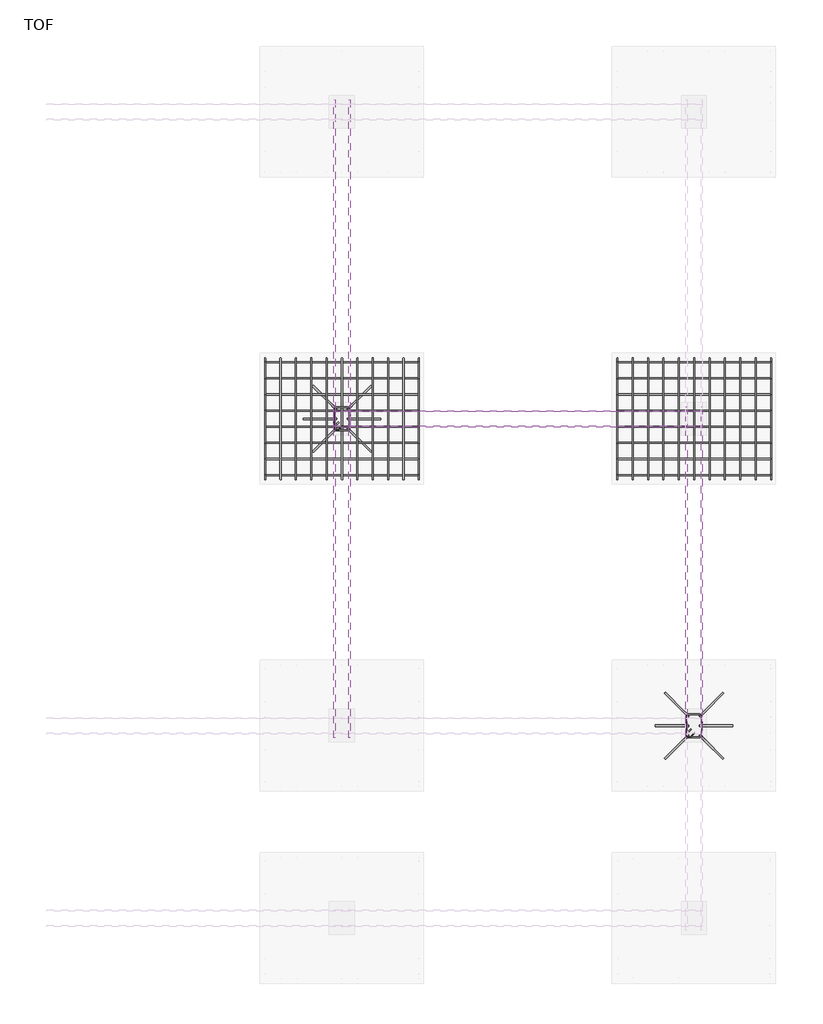
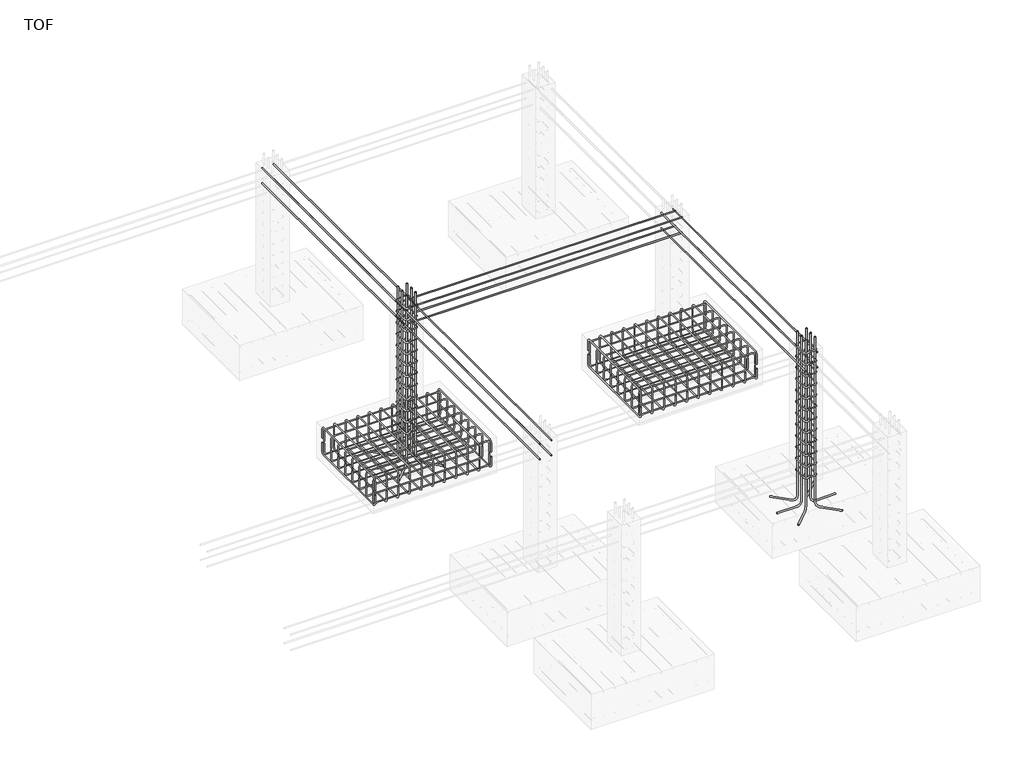
# One storey, part 8 of 10: 38 reinforcing bars.
"""IFC4 building model written with IfcOpenShell, lengths in millimetres."""

from ifc_helpers import new_model, si_unit, point, frame, origin, place, context, project, spatial, polyline, circle_curve, trimmed, segment, composite_curve, source, transform, mapped, element, save
from ifc_brep_helpers import swept_disk

model = new_model("IFC4")

# Units and contexts
model_context = context("Model", 3, world=origin())
ifc_project = project(units=[si_unit("LENGTHUNIT", "METRE", prefix="MILLI")], contexts=[model_context])

# Site, building, storey
site = spatial("IfcSite", under=ifc_project)
building = spatial("IfcBuilding", under=site)
storey = spatial("IfcBuildingStorey", under=building, Name="TOF", Elevation=-1828.8)

# Reinforcing bars
placement = place(None, origin())
reinforcing_bar_shape = source(origin(), model_context, "Body", "SolidModel", [
    swept_disk(composite_curve([segment(polyline([(10345.2782143, -9959.6267376, -2018.8), (10345.2782143, -9959.6267376, -1908.8)]), True, "CONTINUOUS"), segment(trimmed(circle_curve(frame((10345.2782143, -9994.6267376, -1908.8), z_axis=(1.0, 0.0, 0.0), x_axis=(0.0, 35.0, 0.0)), 35.0), [point((10345.2782143, -9959.6267376, -1908.8))], [point((10345.2782143, -9994.6267376, -1873.8))], True, "CARTESIAN"), True, "CONTINUOUS"), segment(polyline([(10345.2782143, -9994.6267376, -1873.8), (10345.2782143, -11034.6267376, -1873.8)]), True, "CONTINUOUS"), segment(trimmed(circle_curve(frame((10345.2782143, -11034.6267376, -1908.8), z_axis=(1.0, 0.0, 0.0), x_axis=(0.0, 0.0, 35.0)), 35.0), [point((10345.2782143, -11034.6267376, -1873.8))], [point((10345.2782143, -11069.6267376, -1908.8))], True, "CARTESIAN"), True, "CONTINUOUS"), segment(polyline([(10345.2782143, -11069.6267376, -1908.8), (10345.2782143, -11069.6267376, -2018.8)]), True, "CONTINUOUS")], self_intersect=False), 5.0),
])
element("IfcReinforcingBar", 1, at=placement, inside=storey, context=model_context, shape_type="MappedRepresentation", body=[
    mapped(reinforcing_bar_shape, transform((0.0, 0.0, 0.0), x_axis=(1.0, 0.0, 0.0), y_axis=(0.0, 1.0, 0.0), z_axis=(0.0, 0.0, 1.0))),
    mapped(reinforcing_bar_shape, transform((-141.0, 0.0, 0.0), x_axis=(1.0, 0.0, 0.0), y_axis=(0.0, 1.0, 0.0), z_axis=(0.0, 0.0, 1.0))),
    mapped(reinforcing_bar_shape, transform((-282.0, 0.0, 0.0), x_axis=(1.0, 0.0, 0.0), y_axis=(0.0, 1.0, 0.0), z_axis=(0.0, 0.0, 1.0))),
    mapped(reinforcing_bar_shape, transform((-423.0, 0.0, 0.0), x_axis=(1.0, 0.0, 0.0), y_axis=(0.0, 1.0, 0.0), z_axis=(0.0, 0.0, 1.0))),
    mapped(reinforcing_bar_shape, transform((-564.0, 0.0, 0.0), x_axis=(1.0, 0.0, 0.0), y_axis=(0.0, 1.0, 0.0), z_axis=(0.0, 0.0, 1.0))),
    mapped(reinforcing_bar_shape, transform((-705.0, 0.0, 0.0), x_axis=(1.0, 0.0, 0.0), y_axis=(0.0, 1.0, 0.0), z_axis=(0.0, 0.0, 1.0))),
    mapped(reinforcing_bar_shape, transform((-846.0, 0.0, 0.0), x_axis=(1.0, 0.0, 0.0), y_axis=(0.0, 1.0, 0.0), z_axis=(0.0, 0.0, 1.0))),
    mapped(reinforcing_bar_shape, transform((-987.0, 0.0, 0.0), x_axis=(1.0, 0.0, 0.0), y_axis=(0.0, 1.0, 0.0), z_axis=(0.0, 0.0, 1.0))),
    mapped(reinforcing_bar_shape, transform((-1128.0, 0.0, 0.0), x_axis=(1.0, 0.0, 0.0), y_axis=(0.0, 1.0, 0.0), z_axis=(0.0, 0.0, 1.0))),
    mapped(reinforcing_bar_shape, transform((-1269.0, 0.0, 0.0), x_axis=(1.0, 0.0, 0.0), y_axis=(0.0, 1.0, 0.0), z_axis=(0.0, 0.0, 1.0))),
    mapped(reinforcing_bar_shape, transform((-1410.0, 0.0, 0.0), x_axis=(1.0, 0.0, 0.0), y_axis=(0.0, 1.0, 0.0), z_axis=(0.0, 0.0, 1.0))),
])
reinforcing_bar_2_shape = source(origin(), model_context, "Body", "SolidModel", [
    swept_disk(composite_curve([segment(polyline([(10345.2782143, -11069.6267376, -2077.5233378), (10345.2782143, -11069.6267376, -2187.5233378)]), True, "CONTINUOUS"), segment(trimmed(circle_curve(frame((10345.2782143, -11034.6267376, -2187.5233378), z_axis=(1.0, 0.0, 0.0), x_axis=(0.0, -35.0, 0.0)), 35.0), [point((10345.2782143, -11069.6267376, -2187.5233378))], [point((10345.2782143, -11034.6267376, -2222.5233378))], True, "CARTESIAN"), True, "CONTINUOUS"), segment(polyline([(10345.2782143, -11034.6267376, -2222.5233378), (10345.2782143, -9994.6267376, -2222.5233378)]), True, "CONTINUOUS"), segment(trimmed(circle_curve(frame((10345.2782143, -9994.6267376, -2187.5233378), z_axis=(1.0, 0.0, 0.0), x_axis=(0.0, 0.0, -35.0)), 35.0), [point((10345.2782143, -9994.6267376, -2222.5233378))], [point((10345.2782143, -9959.6267376, -2187.5233378))], True, "CARTESIAN"), True, "CONTINUOUS"), segment(polyline([(10345.2782143, -9959.6267376, -2187.5233378), (10345.2782143, -9959.6267376, -2077.5233378)]), True, "CONTINUOUS")], self_intersect=False), 5.0),
])
element("IfcReinforcingBar", 2, at=placement, inside=storey, context=model_context, shape_type="MappedRepresentation", body=[
    mapped(reinforcing_bar_2_shape, transform((0.0, 0.0, 0.0), x_axis=(1.0, 0.0, 0.0), y_axis=(0.0, 1.0, 0.0), z_axis=(0.0, 0.0, 1.0))),
    mapped(reinforcing_bar_2_shape, transform((-141.0, 0.0, 0.0), x_axis=(1.0, 0.0, 0.0), y_axis=(0.0, 1.0, 0.0), z_axis=(0.0, 0.0, 1.0))),
    mapped(reinforcing_bar_2_shape, transform((-282.0, 0.0, 0.0), x_axis=(1.0, 0.0, 0.0), y_axis=(0.0, 1.0, 0.0), z_axis=(0.0, 0.0, 1.0))),
    mapped(reinforcing_bar_2_shape, transform((-423.0, 0.0, 0.0), x_axis=(1.0, 0.0, 0.0), y_axis=(0.0, 1.0, 0.0), z_axis=(0.0, 0.0, 1.0))),
    mapped(reinforcing_bar_2_shape, transform((-564.0, 0.0, 0.0), x_axis=(1.0, 0.0, 0.0), y_axis=(0.0, 1.0, 0.0), z_axis=(0.0, 0.0, 1.0))),
    mapped(reinforcing_bar_2_shape, transform((-705.0, 0.0, 0.0), x_axis=(1.0, 0.0, 0.0), y_axis=(0.0, 1.0, 0.0), z_axis=(0.0, 0.0, 1.0))),
    mapped(reinforcing_bar_2_shape, transform((-846.0, 0.0, 0.0), x_axis=(1.0, 0.0, 0.0), y_axis=(0.0, 1.0, 0.0), z_axis=(0.0, 0.0, 1.0))),
    mapped(reinforcing_bar_2_shape, transform((-987.0, 0.0, 0.0), x_axis=(1.0, 0.0, 0.0), y_axis=(0.0, 1.0, 0.0), z_axis=(0.0, 0.0, 1.0))),
    mapped(reinforcing_bar_2_shape, transform((-1128.0, 0.0, 0.0), x_axis=(1.0, 0.0, 0.0), y_axis=(0.0, 1.0, 0.0), z_axis=(0.0, 0.0, 1.0))),
    mapped(reinforcing_bar_2_shape, transform((-1269.0, 0.0, 0.0), x_axis=(1.0, 0.0, 0.0), y_axis=(0.0, 1.0, 0.0), z_axis=(0.0, 0.0, 1.0))),
    mapped(reinforcing_bar_2_shape, transform((-1410.0, 0.0, 0.0), x_axis=(1.0, 0.0, 0.0), y_axis=(0.0, 1.0, 0.0), z_axis=(0.0, 0.0, 1.0))),
])
reinforcing_bar_3_shape = source(origin(), model_context, "Body", "SolidModel", [
    swept_disk(composite_curve([segment(polyline([(10345.2782143, -9994.6861459, -2066.1776706), (10345.2782143, -9994.6861459, -2176.1776706)]), True, "CONTINUOUS"), segment(trimmed(circle_curve(frame((10310.2782143, -9994.6861459, -2176.1776706), z_axis=(0.0, 1.0, 0.0), x_axis=(35.0, 0.0, 0.0)), 35.0), [point((10345.2782143, -9994.6861459, -2176.1776706))], [point((10310.2782143, -9994.6861459, -2211.1776706))], True, "CARTESIAN"), True, "CONTINUOUS"), segment(polyline([(10310.2782143, -9994.6861459, -2211.1776706), (8970.2782143, -9994.6861459, -2211.1776706)]), True, "CONTINUOUS"), segment(trimmed(circle_curve(frame((8970.2782143, -9994.6861459, -2176.1776706), z_axis=(0.0, 1.0, 0.0), x_axis=(0.0, 0.0, -35.0)), 35.0), [point((8970.2782143, -9994.6861459, -2211.1776706))], [point((8935.2782143, -9994.6861459, -2176.1776706))], True, "CARTESIAN"), True, "CONTINUOUS"), segment(polyline([(8935.2782143, -9994.6861459, -2176.1776706), (8935.2782143, -9994.6861459, -2066.1776706)]), True, "CONTINUOUS")], self_intersect=False), 5.0),
])
element("IfcReinforcingBar", 3, at=placement, inside=storey, context=model_context, shape_type="MappedRepresentation", body=[
    mapped(reinforcing_bar_3_shape, transform((0.0, 0.0, 0.0), x_axis=(1.0, 0.0, 0.0), y_axis=(0.0, 1.0, 0.0), z_axis=(0.0, 0.0, 1.0))),
    mapped(reinforcing_bar_3_shape, transform((0.0, -148.0321606, 0.0), x_axis=(1.0, 0.0, 0.0), y_axis=(0.0, 1.0, 0.0), z_axis=(0.0, 0.0, 1.0))),
    mapped(reinforcing_bar_3_shape, transform((0.0, -296.0643211, 0.0), x_axis=(1.0, 0.0, 0.0), y_axis=(0.0, 1.0, 0.0), z_axis=(0.0, 0.0, 1.0))),
    mapped(reinforcing_bar_3_shape, transform((0.0, -444.0964817, 0.0), x_axis=(1.0, 0.0, 0.0), y_axis=(0.0, 1.0, 0.0), z_axis=(0.0, 0.0, 1.0))),
    mapped(reinforcing_bar_3_shape, transform((0.0, -592.1286423, 0.0), x_axis=(1.0, 0.0, 0.0), y_axis=(0.0, 1.0, 0.0), z_axis=(0.0, 0.0, 1.0))),
    mapped(reinforcing_bar_3_shape, transform((0.0, -740.1608029, 0.0), x_axis=(1.0, 0.0, 0.0), y_axis=(0.0, 1.0, 0.0), z_axis=(0.0, 0.0, 1.0))),
    mapped(reinforcing_bar_3_shape, transform((0.0, -888.1929634, 0.0), x_axis=(1.0, 0.0, 0.0), y_axis=(0.0, 1.0, 0.0), z_axis=(0.0, 0.0, 1.0))),
    mapped(reinforcing_bar_3_shape, transform((0.0, -1036.225124, 0.0), x_axis=(1.0, 0.0, 0.0), y_axis=(0.0, 1.0, 0.0), z_axis=(0.0, 0.0, 1.0))),
])
reinforcing_bar_4_shape = source(origin(), model_context, "Body", "SolidModel", [
    swept_disk(composite_curve([segment(polyline([(10345.2782143, -11030.9112699, -2039.256778), (10345.2782143, -11030.9112699, -1929.256778)]), True, "CONTINUOUS"), segment(trimmed(circle_curve(frame((10310.2782143, -11030.9112699, -1929.256778), z_axis=(0.0, -1.0, 0.0), x_axis=(35.0, 0.0, 0.0)), 35.0), [point((10345.2782143, -11030.9112699, -1929.256778))], [point((10310.2782143, -11030.9112699, -1894.256778))], True, "CARTESIAN"), True, "CONTINUOUS"), segment(polyline([(10310.2782143, -11030.9112699, -1894.256778), (8970.2782143, -11030.9112699, -1894.256778)]), True, "CONTINUOUS"), segment(trimmed(circle_curve(frame((8970.2782143, -11030.9112699, -1929.256778), z_axis=(0.0, -1.0, 0.0), x_axis=(0.0, 0.0, 35.0)), 35.0), [point((8970.2782143, -11030.9112699, -1894.256778))], [point((8935.2782143, -11030.9112699, -1929.256778))], True, "CARTESIAN"), True, "CONTINUOUS"), segment(polyline([(8935.2782143, -11030.9112699, -1929.256778), (8935.2782143, -11030.9112699, -2039.256778)]), True, "CONTINUOUS")], self_intersect=False), 5.0),
])
element("IfcReinforcingBar", 4, at=placement, inside=storey, context=model_context, shape_type="MappedRepresentation", body=[
    mapped(reinforcing_bar_4_shape, transform((0.0, 0.0, 0.0), x_axis=(1.0, 0.0, 0.0), y_axis=(0.0, 1.0, 0.0), z_axis=(0.0, 0.0, 1.0))),
    mapped(reinforcing_bar_4_shape, transform((0.0, 148.0321606, 0.0), x_axis=(1.0, 0.0, 0.0), y_axis=(0.0, 1.0, 0.0), z_axis=(0.0, 0.0, 1.0))),
    mapped(reinforcing_bar_4_shape, transform((0.0, 296.0643211, 0.0), x_axis=(1.0, 0.0, 0.0), y_axis=(0.0, 1.0, 0.0), z_axis=(0.0, 0.0, 1.0))),
    mapped(reinforcing_bar_4_shape, transform((0.0, 444.0964817, 0.0), x_axis=(1.0, 0.0, 0.0), y_axis=(0.0, 1.0, 0.0), z_axis=(0.0, 0.0, 1.0))),
    mapped(reinforcing_bar_4_shape, transform((0.0, 592.1286423, 0.0), x_axis=(1.0, 0.0, 0.0), y_axis=(0.0, 1.0, 0.0), z_axis=(0.0, 0.0, 1.0))),
    mapped(reinforcing_bar_4_shape, transform((0.0, 740.1608029, 0.0), x_axis=(1.0, 0.0, 0.0), y_axis=(0.0, 1.0, 0.0), z_axis=(0.0, 0.0, 1.0))),
    mapped(reinforcing_bar_4_shape, transform((0.0, 888.1929634, 0.0), x_axis=(1.0, 0.0, 0.0), y_axis=(0.0, 1.0, 0.0), z_axis=(0.0, 0.0, 1.0))),
    mapped(reinforcing_bar_4_shape, transform((0.0, 1036.225124, 0.0), x_axis=(1.0, 0.0, 0.0), y_axis=(0.0, 1.0, 0.0), z_axis=(0.0, 0.0, 1.0))),
])
reinforcing_bar_5_shape = source(origin(), model_context, "Body", "SolidModel", [
    swept_disk(composite_curve([segment(polyline([(13575.2782143, -9959.6267376, -2018.8), (13575.2782143, -9959.6267376, -1908.8)]), True, "CONTINUOUS"), segment(trimmed(circle_curve(frame((13575.2782143, -9994.6267376, -1908.8), z_axis=(1.0, 0.0, 0.0), x_axis=(0.0, 35.0, 0.0)), 35.0), [point((13575.2782143, -9959.6267376, -1908.8))], [point((13575.2782143, -9994.6267376, -1873.8))], True, "CARTESIAN"), True, "CONTINUOUS"), segment(polyline([(13575.2782143, -9994.6267376, -1873.8), (13575.2782143, -11034.6267376, -1873.8)]), True, "CONTINUOUS"), segment(trimmed(circle_curve(frame((13575.2782143, -11034.6267376, -1908.8), z_axis=(1.0, 0.0, 0.0), x_axis=(0.0, 0.0, 35.0)), 35.0), [point((13575.2782143, -11034.6267376, -1873.8))], [point((13575.2782143, -11069.6267376, -1908.8))], True, "CARTESIAN"), True, "CONTINUOUS"), segment(polyline([(13575.2782143, -11069.6267376, -1908.8), (13575.2782143, -11069.6267376, -2018.8)]), True, "CONTINUOUS")], self_intersect=False), 5.0),
])
element("IfcReinforcingBar", 5, at=placement, inside=storey, context=model_context, shape_type="MappedRepresentation", body=[
    mapped(reinforcing_bar_5_shape, transform((0.0, 0.0, 0.0), x_axis=(1.0, 0.0, 0.0), y_axis=(0.0, 1.0, 0.0), z_axis=(0.0, 0.0, 1.0))),
    mapped(reinforcing_bar_5_shape, transform((-141.0, 0.0, 0.0), x_axis=(1.0, 0.0, 0.0), y_axis=(0.0, 1.0, 0.0), z_axis=(0.0, 0.0, 1.0))),
    mapped(reinforcing_bar_5_shape, transform((-282.0, 0.0, 0.0), x_axis=(1.0, 0.0, 0.0), y_axis=(0.0, 1.0, 0.0), z_axis=(0.0, 0.0, 1.0))),
    mapped(reinforcing_bar_5_shape, transform((-423.0, 0.0, 0.0), x_axis=(1.0, 0.0, 0.0), y_axis=(0.0, 1.0, 0.0), z_axis=(0.0, 0.0, 1.0))),
    mapped(reinforcing_bar_5_shape, transform((-564.0, 0.0, 0.0), x_axis=(1.0, 0.0, 0.0), y_axis=(0.0, 1.0, 0.0), z_axis=(0.0, 0.0, 1.0))),
    mapped(reinforcing_bar_5_shape, transform((-705.0, 0.0, 0.0), x_axis=(1.0, 0.0, 0.0), y_axis=(0.0, 1.0, 0.0), z_axis=(0.0, 0.0, 1.0))),
    mapped(reinforcing_bar_5_shape, transform((-846.0, 0.0, 0.0), x_axis=(1.0, 0.0, 0.0), y_axis=(0.0, 1.0, 0.0), z_axis=(0.0, 0.0, 1.0))),
    mapped(reinforcing_bar_5_shape, transform((-987.0, 0.0, 0.0), x_axis=(1.0, 0.0, 0.0), y_axis=(0.0, 1.0, 0.0), z_axis=(0.0, 0.0, 1.0))),
    mapped(reinforcing_bar_5_shape, transform((-1128.0, 0.0, 0.0), x_axis=(1.0, 0.0, 0.0), y_axis=(0.0, 1.0, 0.0), z_axis=(0.0, 0.0, 1.0))),
    mapped(reinforcing_bar_5_shape, transform((-1269.0, 0.0, 0.0), x_axis=(1.0, 0.0, 0.0), y_axis=(0.0, 1.0, 0.0), z_axis=(0.0, 0.0, 1.0))),
    mapped(reinforcing_bar_5_shape, transform((-1410.0, 0.0, 0.0), x_axis=(1.0, 0.0, 0.0), y_axis=(0.0, 1.0, 0.0), z_axis=(0.0, 0.0, 1.0))),
])
reinforcing_bar_6_shape = source(origin(), model_context, "Body", "SolidModel", [
    swept_disk(composite_curve([segment(polyline([(13575.2782143, -11069.6267376, -2077.5233378), (13575.2782143, -11069.6267376, -2187.5233378)]), True, "CONTINUOUS"), segment(trimmed(circle_curve(frame((13575.2782143, -11034.6267376, -2187.5233378), z_axis=(1.0, 0.0, 0.0), x_axis=(0.0, -35.0, 0.0)), 35.0), [point((13575.2782143, -11069.6267376, -2187.5233378))], [point((13575.2782143, -11034.6267376, -2222.5233378))], True, "CARTESIAN"), True, "CONTINUOUS"), segment(polyline([(13575.2782143, -11034.6267376, -2222.5233378), (13575.2782143, -9994.6267376, -2222.5233378)]), True, "CONTINUOUS"), segment(trimmed(circle_curve(frame((13575.2782143, -9994.6267376, -2187.5233378), z_axis=(1.0, 0.0, 0.0), x_axis=(0.0, 0.0, -35.0)), 35.0), [point((13575.2782143, -9994.6267376, -2222.5233378))], [point((13575.2782143, -9959.6267376, -2187.5233378))], True, "CARTESIAN"), True, "CONTINUOUS"), segment(polyline([(13575.2782143, -9959.6267376, -2187.5233378), (13575.2782143, -9959.6267376, -2077.5233378)]), True, "CONTINUOUS")], self_intersect=False), 5.0),
])
element("IfcReinforcingBar", 6, at=placement, inside=storey, context=model_context, shape_type="MappedRepresentation", body=[
    mapped(reinforcing_bar_6_shape, transform((0.0, 0.0, 0.0), x_axis=(1.0, 0.0, 0.0), y_axis=(0.0, 1.0, 0.0), z_axis=(0.0, 0.0, 1.0))),
    mapped(reinforcing_bar_6_shape, transform((-141.0, 0.0, 0.0), x_axis=(1.0, 0.0, 0.0), y_axis=(0.0, 1.0, 0.0), z_axis=(0.0, 0.0, 1.0))),
    mapped(reinforcing_bar_6_shape, transform((-282.0, 0.0, 0.0), x_axis=(1.0, 0.0, 0.0), y_axis=(0.0, 1.0, 0.0), z_axis=(0.0, 0.0, 1.0))),
    mapped(reinforcing_bar_6_shape, transform((-423.0, 0.0, 0.0), x_axis=(1.0, 0.0, 0.0), y_axis=(0.0, 1.0, 0.0), z_axis=(0.0, 0.0, 1.0))),
    mapped(reinforcing_bar_6_shape, transform((-564.0, 0.0, 0.0), x_axis=(1.0, 0.0, 0.0), y_axis=(0.0, 1.0, 0.0), z_axis=(0.0, 0.0, 1.0))),
    mapped(reinforcing_bar_6_shape, transform((-705.0, 0.0, 0.0), x_axis=(1.0, 0.0, 0.0), y_axis=(0.0, 1.0, 0.0), z_axis=(0.0, 0.0, 1.0))),
    mapped(reinforcing_bar_6_shape, transform((-846.0, 0.0, 0.0), x_axis=(1.0, 0.0, 0.0), y_axis=(0.0, 1.0, 0.0), z_axis=(0.0, 0.0, 1.0))),
    mapped(reinforcing_bar_6_shape, transform((-987.0, 0.0, 0.0), x_axis=(1.0, 0.0, 0.0), y_axis=(0.0, 1.0, 0.0), z_axis=(0.0, 0.0, 1.0))),
    mapped(reinforcing_bar_6_shape, transform((-1128.0, 0.0, 0.0), x_axis=(1.0, 0.0, 0.0), y_axis=(0.0, 1.0, 0.0), z_axis=(0.0, 0.0, 1.0))),
    mapped(reinforcing_bar_6_shape, transform((-1269.0, 0.0, 0.0), x_axis=(1.0, 0.0, 0.0), y_axis=(0.0, 1.0, 0.0), z_axis=(0.0, 0.0, 1.0))),
    mapped(reinforcing_bar_6_shape, transform((-1410.0, 0.0, 0.0), x_axis=(1.0, 0.0, 0.0), y_axis=(0.0, 1.0, 0.0), z_axis=(0.0, 0.0, 1.0))),
])
reinforcing_bar_7_shape = source(origin(), model_context, "Body", "SolidModel", [
    swept_disk(composite_curve([segment(polyline([(13575.2782143, -9994.6861459, -2066.1776706), (13575.2782143, -9994.6861459, -2176.1776706)]), True, "CONTINUOUS"), segment(trimmed(circle_curve(frame((13540.2782143, -9994.6861459, -2176.1776706), z_axis=(0.0, 1.0, 0.0), x_axis=(35.0, 0.0, 0.0)), 35.0), [point((13575.2782143, -9994.6861459, -2176.1776706))], [point((13540.2782143, -9994.6861459, -2211.1776706))], True, "CARTESIAN"), True, "CONTINUOUS"), segment(polyline([(13540.2782143, -9994.6861459, -2211.1776706), (12200.2782143, -9994.6861459, -2211.1776706)]), True, "CONTINUOUS"), segment(trimmed(circle_curve(frame((12200.2782143, -9994.6861459, -2176.1776706), z_axis=(0.0, 1.0, 0.0), x_axis=(0.0, 0.0, -35.0)), 35.0), [point((12200.2782143, -9994.6861459, -2211.1776706))], [point((12165.2782143, -9994.6861459, -2176.1776706))], True, "CARTESIAN"), True, "CONTINUOUS"), segment(polyline([(12165.2782143, -9994.6861459, -2176.1776706), (12165.2782143, -9994.6861459, -2066.1776706)]), True, "CONTINUOUS")], self_intersect=False), 5.0),
])
element("IfcReinforcingBar", 7, at=placement, inside=storey, context=model_context, shape_type="MappedRepresentation", body=[
    mapped(reinforcing_bar_7_shape, transform((0.0, 0.0, 0.0), x_axis=(1.0, 0.0, 0.0), y_axis=(0.0, 1.0, 0.0), z_axis=(0.0, 0.0, 1.0))),
    mapped(reinforcing_bar_7_shape, transform((0.0, -148.0321606, 0.0), x_axis=(1.0, 0.0, 0.0), y_axis=(0.0, 1.0, 0.0), z_axis=(0.0, 0.0, 1.0))),
    mapped(reinforcing_bar_7_shape, transform((0.0, -296.0643211, 0.0), x_axis=(1.0, 0.0, 0.0), y_axis=(0.0, 1.0, 0.0), z_axis=(0.0, 0.0, 1.0))),
    mapped(reinforcing_bar_7_shape, transform((0.0, -444.0964817, 0.0), x_axis=(1.0, 0.0, 0.0), y_axis=(0.0, 1.0, 0.0), z_axis=(0.0, 0.0, 1.0))),
    mapped(reinforcing_bar_7_shape, transform((0.0, -592.1286423, 0.0), x_axis=(1.0, 0.0, 0.0), y_axis=(0.0, 1.0, 0.0), z_axis=(0.0, 0.0, 1.0))),
    mapped(reinforcing_bar_7_shape, transform((0.0, -740.1608029, 0.0), x_axis=(1.0, 0.0, 0.0), y_axis=(0.0, 1.0, 0.0), z_axis=(0.0, 0.0, 1.0))),
    mapped(reinforcing_bar_7_shape, transform((0.0, -888.1929634, 0.0), x_axis=(1.0, 0.0, 0.0), y_axis=(0.0, 1.0, 0.0), z_axis=(0.0, 0.0, 1.0))),
    mapped(reinforcing_bar_7_shape, transform((0.0, -1036.225124, 0.0), x_axis=(1.0, 0.0, 0.0), y_axis=(0.0, 1.0, 0.0), z_axis=(0.0, 0.0, 1.0))),
])
reinforcing_bar_8_shape = source(origin(), model_context, "Body", "SolidModel", [
    swept_disk(composite_curve([segment(polyline([(13575.2782143, -11030.9112699, -2039.256778), (13575.2782143, -11030.9112699, -1929.256778)]), True, "CONTINUOUS"), segment(trimmed(circle_curve(frame((13540.2782143, -11030.9112699, -1929.256778), z_axis=(0.0, -1.0, 0.0), x_axis=(35.0, 0.0, 0.0)), 35.0), [point((13575.2782143, -11030.9112699, -1929.256778))], [point((13540.2782143, -11030.9112699, -1894.256778))], True, "CARTESIAN"), True, "CONTINUOUS"), segment(polyline([(13540.2782143, -11030.9112699, -1894.256778), (12200.2782143, -11030.9112699, -1894.256778)]), True, "CONTINUOUS"), segment(trimmed(circle_curve(frame((12200.2782143, -11030.9112699, -1929.256778), z_axis=(0.0, -1.0, 0.0), x_axis=(0.0, 0.0, 35.0)), 35.0), [point((12200.2782143, -11030.9112699, -1894.256778))], [point((12165.2782143, -11030.9112699, -1929.256778))], True, "CARTESIAN"), True, "CONTINUOUS"), segment(polyline([(12165.2782143, -11030.9112699, -1929.256778), (12165.2782143, -11030.9112699, -2039.256778)]), True, "CONTINUOUS")], self_intersect=False), 5.0),
])
element("IfcReinforcingBar", 8, at=placement, inside=storey, context=model_context, shape_type="MappedRepresentation", body=[
    mapped(reinforcing_bar_8_shape, transform((0.0, 0.0, 0.0), x_axis=(1.0, 0.0, 0.0), y_axis=(0.0, 1.0, 0.0), z_axis=(0.0, 0.0, 1.0))),
    mapped(reinforcing_bar_8_shape, transform((0.0, 148.0321606, 0.0), x_axis=(1.0, 0.0, 0.0), y_axis=(0.0, 1.0, 0.0), z_axis=(0.0, 0.0, 1.0))),
    mapped(reinforcing_bar_8_shape, transform((0.0, 296.0643211, 0.0), x_axis=(1.0, 0.0, 0.0), y_axis=(0.0, 1.0, 0.0), z_axis=(0.0, 0.0, 1.0))),
    mapped(reinforcing_bar_8_shape, transform((0.0, 444.0964817, 0.0), x_axis=(1.0, 0.0, 0.0), y_axis=(0.0, 1.0, 0.0), z_axis=(0.0, 0.0, 1.0))),
    mapped(reinforcing_bar_8_shape, transform((0.0, 592.1286423, 0.0), x_axis=(1.0, 0.0, 0.0), y_axis=(0.0, 1.0, 0.0), z_axis=(0.0, 0.0, 1.0))),
    mapped(reinforcing_bar_8_shape, transform((0.0, 740.1608029, 0.0), x_axis=(1.0, 0.0, 0.0), y_axis=(0.0, 1.0, 0.0), z_axis=(0.0, 0.0, 1.0))),
    mapped(reinforcing_bar_8_shape, transform((0.0, 888.1929634, 0.0), x_axis=(1.0, 0.0, 0.0), y_axis=(0.0, 1.0, 0.0), z_axis=(0.0, 0.0, 1.0))),
    mapped(reinforcing_bar_8_shape, transform((0.0, 1036.225124, 0.0), x_axis=(1.0, 0.0, 0.0), y_axis=(0.0, 1.0, 0.0), z_axis=(0.0, 0.0, 1.0))),
])
reinforcing_bar_9_shape = source(origin(), model_context, "Body", "SolidModel", [
    swept_disk(composite_curve([segment(polyline([(12840.248777, -13360.7150493, -1784.8), (12806.3076515, -13394.6561748, -1784.8)]), True, "CONTINUOUS"), segment(trimmed(circle_curve(frame((12823.2782143, -13411.6267376, -1784.8), z_axis=(0.0, 0.0, 1.0), x_axis=(-16.970562800001062, 16.970562799999243, 0.0)), 24.0), [point((12806.3076515, -13394.6561748, -1784.8))], [point((12823.2782143, -13435.6267376, -1784.8))], True, "CARTESIAN"), True, "CONTINUOUS"), segment(polyline([(12823.2782143, -13435.6267376, -1784.8), (12917.2782143, -13435.6267376, -1784.8)]), True, "CONTINUOUS"), segment(trimmed(circle_curve(frame((12917.2782143, -13411.6267376, -1784.8), z_axis=(0.0, 0.0, 1.0), x_axis=(0.0, -24.0, 0.0)), 24.0), [point((12917.2782143, -13435.6267376, -1784.8))], [point((12941.2782143, -13411.6267376, -1784.8))], True, "CARTESIAN"), True, "CONTINUOUS"), segment(polyline([(12941.2782143, -13411.6267376, -1784.8), (12941.2782143, -13247.6267376, -1784.8)]), True, "CONTINUOUS"), segment(trimmed(circle_curve(frame((12917.3162115, -13247.6267376, -1786.149972), z_axis=(-0.05624883273897078, 0.0, 0.9984167811167355), x_axis=(23.962002800000846, 0.0, 1.3499719999999797)), 24.0), [point((12941.2782143, -13247.6267376, -1784.8))], [point((12917.3162115, -13223.6267376, -1786.149972))], True, "CARTESIAN"), True, "CONTINUOUS"), segment(polyline([(12917.3162115, -13223.6267376, -1786.149972), (12823.240217, -13223.6267376, -1791.450028)]), True, "CONTINUOUS"), segment(trimmed(circle_curve(frame((12823.240217, -13247.6267376, -1791.450028), z_axis=(-0.05624883273897078, 0.0, 0.9984167811167355), x_axis=(0.0, 24.0, 0.0)), 24.0), [point((12823.240217, -13223.6267376, -1791.450028))], [point((12799.2782143, -13247.6267376, -1792.8))], True, "CARTESIAN"), True, "CONTINUOUS"), segment(polyline([(12799.2782143, -13247.6267376, -1792.8), (12799.2782143, -13411.6267376, -1792.8)]), True, "CONTINUOUS"), segment(trimmed(circle_curve(frame((12823.2782143, -13411.6267376, -1792.8), z_axis=(0.0, 0.0, 1.0), x_axis=(-24.0, 0.0, 0.0)), 24.0), [point((12799.2782143, -13411.6267376, -1792.8))], [point((12840.248777, -13428.5973003, -1792.8))], True, "CARTESIAN"), True, "CONTINUOUS"), segment(polyline([(12840.248777, -13428.5973003, -1792.8), (12874.1899025, -13394.6561748, -1792.8)]), True, "CONTINUOUS")], self_intersect=False), 4.0),
])
element("IfcReinforcingBar", 9, at=placement, inside=storey, context=model_context, shape_type="MappedRepresentation", body=[
    mapped(reinforcing_bar_9_shape, transform((0.0, 0.0, 0.0), x_axis=(1.0, 0.0, 0.0), y_axis=(0.0, 1.0, 0.0), z_axis=(0.0, 0.0, 1.0))),
    mapped(reinforcing_bar_9_shape, transform((0.0, 0.0, 145.9395608), x_axis=(1.0, 0.0, 0.0), y_axis=(0.0, 1.0, 0.0), z_axis=(0.0, 0.0, 1.0))),
    mapped(reinforcing_bar_9_shape, transform((0.0, 0.0, 291.8791216), x_axis=(1.0, 0.0, 0.0), y_axis=(0.0, 1.0, 0.0), z_axis=(0.0, 0.0, 1.0))),
    mapped(reinforcing_bar_9_shape, transform((0.0, 0.0, 437.8186825), x_axis=(1.0, 0.0, 0.0), y_axis=(0.0, 1.0, 0.0), z_axis=(0.0, 0.0, 1.0))),
    mapped(reinforcing_bar_9_shape, transform((0.0, 0.0, 583.7582433), x_axis=(1.0, 0.0, 0.0), y_axis=(0.0, 1.0, 0.0), z_axis=(0.0, 0.0, 1.0))),
    mapped(reinforcing_bar_9_shape, transform((0.0, 0.0, 729.6978041), x_axis=(1.0, 0.0, 0.0), y_axis=(0.0, 1.0, 0.0), z_axis=(0.0, 0.0, 1.0))),
    mapped(reinforcing_bar_9_shape, transform((0.0, 0.0, 875.6373649), x_axis=(1.0, 0.0, 0.0), y_axis=(0.0, 1.0, 0.0), z_axis=(0.0, 0.0, 1.0))),
    mapped(reinforcing_bar_9_shape, transform((0.0, 0.0, 1021.5769258), x_axis=(1.0, 0.0, 0.0), y_axis=(0.0, 1.0, 0.0), z_axis=(0.0, 0.0, 1.0))),
    mapped(reinforcing_bar_9_shape, transform((0.0, 0.0, 1167.5164866), x_axis=(1.0, 0.0, 0.0), y_axis=(0.0, 1.0, 0.0), z_axis=(0.0, 0.0, 1.0))),
    mapped(reinforcing_bar_9_shape, transform((0.0, 0.0, 1313.4560474), x_axis=(1.0, 0.0, 0.0), y_axis=(0.0, 1.0, 0.0), z_axis=(0.0, 0.0, 1.0))),
    mapped(reinforcing_bar_9_shape, transform((0.0, 0.0, 1459.3956082), x_axis=(1.0, 0.0, 0.0), y_axis=(0.0, 1.0, 0.0), z_axis=(0.0, 0.0, 1.0))),
    mapped(reinforcing_bar_9_shape, transform((0.0, 0.0, 1605.3351691), x_axis=(1.0, 0.0, 0.0), y_axis=(0.0, 1.0, 0.0), z_axis=(0.0, 0.0, 1.0))),
])
element("IfcReinforcingBar", 10, at=placement, inside=storey, context=model_context, shape_type="SolidModel", body=[
    swept_disk(composite_curve([segment(polyline([(12925.884816, -13420.2333393, -20.0), (12925.884816, -13420.2333393, -2138.7824747)]), True, "CONTINUOUS"), segment(trimmed(circle_curve(frame((12965.1292424, -13459.4777657, -2138.7824747), z_axis=(-0.7071067811865545, -0.7071067811865406, 0.0), x_axis=(-39.24442640000052, 39.2444263999987, 0.0)), 55.5), [point((12925.884816, -13420.2333393, -2138.7824747))], [point((12965.1292424, -13459.4777657, -2194.2824747))], True, "CARTESIAN"), True, "CONTINUOUS"), segment(polyline([(12965.1292424, -13459.4777657, -2194.2824747), (13137.5083915, -13631.8569148, -2194.2824747)]), True, "CONTINUOUS")], self_intersect=False), 8.0),
])
element("IfcReinforcingBar", 11, at=placement, inside=storey, context=model_context, shape_type="SolidModel", body=[
    swept_disk(composite_curve([segment(polyline([(12925.934816, -13329.6267376, -20.0), (12925.934816, -13329.6267376, -2138.7824747)]), True, "CONTINUOUS"), segment(trimmed(circle_curve(frame((12981.434816, -13329.6267376, -2138.7824747), z_axis=(0.0, -1.0, 0.0), x_axis=(-55.5, 0.0, 0.0)), 55.5), [point((12925.934816, -13329.6267376, -2138.7824747))], [point((12981.434816, -13329.6267376, -2194.2824747))], True, "CARTESIAN"), True, "CONTINUOUS"), segment(polyline([(12981.434816, -13329.6267376, -2194.2824747), (13225.1657466, -13329.6267376, -2194.2824747)]), True, "CONTINUOUS")], self_intersect=False), 8.0),
])
element("IfcReinforcingBar", 12, at=placement, inside=storey, context=model_context, shape_type="SolidModel", body=[
    swept_disk(composite_curve([segment(polyline([(12925.884816, -13239.0201359, -20.0), (12925.884816, -13239.0201359, -2138.7824747)]), True, "CONTINUOUS"), segment(trimmed(circle_curve(frame((12965.1292424, -13199.7757095, -2138.7824747), z_axis=(0.7071067811865545, -0.7071067811865407, 0.0), x_axis=(-39.24442640000052, -39.24442640000052, 0.0)), 55.5), [point((12925.884816, -13239.0201359, -2138.7824747))], [point((12965.1292424, -13199.7757095, -2194.2824747))], True, "CARTESIAN"), True, "CONTINUOUS"), segment(polyline([(12965.1292424, -13199.7757095, -2194.2824747), (13137.5083915, -13027.3965603, -2194.2824747)]), True, "CONTINUOUS")], self_intersect=False), 8.0),
])
element("IfcReinforcingBar", 13, at=placement, inside=storey, context=model_context, shape_type="SolidModel", body=[
    swept_disk(composite_curve([segment(polyline([(12814.6716126, -13420.2333393, -20.0), (12814.6716126, -13420.2333393, -2138.7824747)]), True, "CONTINUOUS"), segment(trimmed(circle_curve(frame((12775.4271862, -13459.4777657, -2138.7824747), z_axis=(-0.7071067811865517, 0.7071067811865434, 0.0), x_axis=(39.2444263999987, 39.2444263999987, 0.0)), 55.5), [point((12814.6716126, -13420.2333393, -2138.7824747))], [point((12775.4271862, -13459.4777657, -2194.2824747))], True, "CARTESIAN"), True, "CONTINUOUS"), segment(polyline([(12775.4271862, -13459.4777657, -2194.2824747), (12603.048037, -13631.8569148, -2194.2824747)]), True, "CONTINUOUS")], self_intersect=False), 8.0),
])
element("IfcReinforcingBar", 14, at=placement, inside=storey, context=model_context, shape_type="SolidModel", body=[
    swept_disk(composite_curve([segment(polyline([(12814.6216126, -13329.6267376, -20.0), (12814.6216126, -13329.6267376, -2138.7824747)]), True, "CONTINUOUS"), segment(trimmed(circle_curve(frame((12759.1216126, -13329.6267376, -2138.7824747), z_axis=(0.0, 1.0, 0.0), x_axis=(55.5, 0.0, 0.0)), 55.5), [point((12814.6216126, -13329.6267376, -2138.7824747))], [point((12759.1216126, -13329.6267376, -2194.2824747))], True, "CARTESIAN"), True, "CONTINUOUS"), segment(polyline([(12759.1216126, -13329.6267376, -2194.2824747), (12515.3906819, -13329.6267376, -2194.2824747)]), True, "CONTINUOUS")], self_intersect=False), 8.0),
])
element("IfcReinforcingBar", 15, at=placement, inside=storey, context=model_context, shape_type="SolidModel", body=[
    swept_disk(composite_curve([segment(polyline([(12814.6716126, -13239.0201359, -20.0), (12814.6716126, -13239.0201359, -2138.7824747)]), True, "CONTINUOUS"), segment(trimmed(circle_curve(frame((12775.4271862, -13199.7757095, -2138.7824747), z_axis=(0.7071067811865572, 0.7071067811865379, 0.0), x_axis=(39.2444263999987, -39.24442640000052, 0.0)), 55.5), [point((12814.6716126, -13239.0201359, -2138.7824747))], [point((12775.4271862, -13199.7757095, -2194.2824747))], True, "CARTESIAN"), True, "CONTINUOUS"), segment(polyline([(12775.4271862, -13199.7757095, -2194.2824747), (12603.048037, -13027.3965603, -2194.2824747)]), True, "CONTINUOUS")], self_intersect=False), 8.0),
])
reinforcing_bar_10_shape = source(origin(), model_context, "Body", "SolidModel", [
    swept_disk(composite_curve([segment(polyline([(9610.248777, -10545.7150493, -1784.8), (9576.3076515, -10579.6561748, -1784.8)]), True, "CONTINUOUS"), segment(trimmed(circle_curve(frame((9593.2782143, -10596.6267376, -1784.8), z_axis=(0.0, 0.0, 1.0), x_axis=(-16.970562800001062, 16.970562799999243, 0.0)), 24.0), [point((9576.3076515, -10579.6561748, -1784.8))], [point((9593.2782143, -10620.6267376, -1784.8))], True, "CARTESIAN"), True, "CONTINUOUS"), segment(polyline([(9593.2782143, -10620.6267376, -1784.8), (9687.2782143, -10620.6267376, -1784.8)]), True, "CONTINUOUS"), segment(trimmed(circle_curve(frame((9687.2782143, -10596.6267376, -1784.8), z_axis=(0.0, 0.0, 1.0), x_axis=(0.0, -24.0, 0.0)), 24.0), [point((9687.2782143, -10620.6267376, -1784.8))], [point((9711.2782143, -10596.6267376, -1784.8))], True, "CARTESIAN"), True, "CONTINUOUS"), segment(polyline([(9711.2782143, -10596.6267376, -1784.8), (9711.2782143, -10432.6267376, -1784.8)]), True, "CONTINUOUS"), segment(trimmed(circle_curve(frame((9687.3162115, -10432.6267376, -1786.149972), z_axis=(-0.05624883273897078, 0.0, 0.9984167811167355), x_axis=(23.962002800000846, 0.0, 1.3499719999999797)), 24.0), [point((9711.2782143, -10432.6267376, -1784.8))], [point((9687.3162115, -10408.6267376, -1786.149972))], True, "CARTESIAN"), True, "CONTINUOUS"), segment(polyline([(9687.3162115, -10408.6267376, -1786.149972), (9593.240217, -10408.6267376, -1791.450028)]), True, "CONTINUOUS"), segment(trimmed(circle_curve(frame((9593.240217, -10432.6267376, -1791.450028), z_axis=(-0.05624883273897078, 0.0, 0.9984167811167355), x_axis=(0.0, 24.0, 0.0)), 24.0), [point((9593.240217, -10408.6267376, -1791.450028))], [point((9569.2782143, -10432.6267376, -1792.8))], True, "CARTESIAN"), True, "CONTINUOUS"), segment(polyline([(9569.2782143, -10432.6267376, -1792.8), (9569.2782143, -10596.6267376, -1792.8)]), True, "CONTINUOUS"), segment(trimmed(circle_curve(frame((9593.2782143, -10596.6267376, -1792.8), z_axis=(0.0, 0.0, 1.0), x_axis=(-24.0, 0.0, 0.0)), 24.0), [point((9569.2782143, -10596.6267376, -1792.8))], [point((9610.248777, -10613.5973003, -1792.8))], True, "CARTESIAN"), True, "CONTINUOUS"), segment(polyline([(9610.248777, -10613.5973003, -1792.8), (9644.1899025, -10579.6561748, -1792.8)]), True, "CONTINUOUS")], self_intersect=False), 4.0),
])
element("IfcReinforcingBar", 16, at=placement, inside=storey, context=model_context, shape_type="MappedRepresentation", body=[
    mapped(reinforcing_bar_10_shape, transform((0.0, 0.0, 0.0), x_axis=(1.0, 0.0, 0.0), y_axis=(0.0, 1.0, 0.0), z_axis=(0.0, 0.0, 1.0))),
    mapped(reinforcing_bar_10_shape, transform((0.0, 0.0, 145.9395608), x_axis=(1.0, 0.0, 0.0), y_axis=(0.0, 1.0, 0.0), z_axis=(0.0, 0.0, 1.0))),
    mapped(reinforcing_bar_10_shape, transform((0.0, 0.0, 291.8791216), x_axis=(1.0, 0.0, 0.0), y_axis=(0.0, 1.0, 0.0), z_axis=(0.0, 0.0, 1.0))),
    mapped(reinforcing_bar_10_shape, transform((0.0, 0.0, 437.8186825), x_axis=(1.0, 0.0, 0.0), y_axis=(0.0, 1.0, 0.0), z_axis=(0.0, 0.0, 1.0))),
    mapped(reinforcing_bar_10_shape, transform((0.0, 0.0, 583.7582433), x_axis=(1.0, 0.0, 0.0), y_axis=(0.0, 1.0, 0.0), z_axis=(0.0, 0.0, 1.0))),
    mapped(reinforcing_bar_10_shape, transform((0.0, 0.0, 729.6978041), x_axis=(1.0, 0.0, 0.0), y_axis=(0.0, 1.0, 0.0), z_axis=(0.0, 0.0, 1.0))),
    mapped(reinforcing_bar_10_shape, transform((0.0, 0.0, 875.6373649), x_axis=(1.0, 0.0, 0.0), y_axis=(0.0, 1.0, 0.0), z_axis=(0.0, 0.0, 1.0))),
    mapped(reinforcing_bar_10_shape, transform((0.0, 0.0, 1021.5769258), x_axis=(1.0, 0.0, 0.0), y_axis=(0.0, 1.0, 0.0), z_axis=(0.0, 0.0, 1.0))),
    mapped(reinforcing_bar_10_shape, transform((0.0, 0.0, 1167.5164866), x_axis=(1.0, 0.0, 0.0), y_axis=(0.0, 1.0, 0.0), z_axis=(0.0, 0.0, 1.0))),
    mapped(reinforcing_bar_10_shape, transform((0.0, 0.0, 1313.4560474), x_axis=(1.0, 0.0, 0.0), y_axis=(0.0, 1.0, 0.0), z_axis=(0.0, 0.0, 1.0))),
    mapped(reinforcing_bar_10_shape, transform((0.0, 0.0, 1459.3956082), x_axis=(1.0, 0.0, 0.0), y_axis=(0.0, 1.0, 0.0), z_axis=(0.0, 0.0, 1.0))),
    mapped(reinforcing_bar_10_shape, transform((0.0, 0.0, 1605.3351691), x_axis=(1.0, 0.0, 0.0), y_axis=(0.0, 1.0, 0.0), z_axis=(0.0, 0.0, 1.0))),
])
element("IfcReinforcingBar", 17, at=placement, inside=storey, context=model_context, shape_type="SolidModel", body=[
    swept_disk(composite_curve([segment(polyline([(9695.884816, -10605.2333393, -20.0), (9695.884816, -10605.2333393, -2138.7824747)]), True, "CONTINUOUS"), segment(trimmed(circle_curve(frame((9735.1292424, -10644.4777657, -2138.7824747), z_axis=(-0.7071067811865545, -0.7071067811865406, 0.0), x_axis=(-39.24442640000052, 39.2444263999987, 0.0)), 55.5), [point((9695.884816, -10605.2333393, -2138.7824747))], [point((9735.1292424, -10644.4777657, -2194.2824747))], True, "CARTESIAN"), True, "CONTINUOUS"), segment(polyline([(9735.1292424, -10644.4777657, -2194.2824747), (9907.5083915, -10816.8569148, -2194.2824747)]), True, "CONTINUOUS")], self_intersect=False), 8.0),
])
element("IfcReinforcingBar", 18, at=placement, inside=storey, context=model_context, shape_type="SolidModel", body=[
    swept_disk(composite_curve([segment(polyline([(9695.934816, -10514.6267376, -20.0), (9695.934816, -10514.6267376, -2138.7824747)]), True, "CONTINUOUS"), segment(trimmed(circle_curve(frame((9751.434816, -10514.6267376, -2138.7824747), z_axis=(0.0, -1.0, 0.0), x_axis=(-55.5, 0.0, 0.0)), 55.5), [point((9695.934816, -10514.6267376, -2138.7824747))], [point((9751.434816, -10514.6267376, -2194.2824747))], True, "CARTESIAN"), True, "CONTINUOUS"), segment(polyline([(9751.434816, -10514.6267376, -2194.2824747), (9995.1657466, -10514.6267376, -2194.2824747)]), True, "CONTINUOUS")], self_intersect=False), 8.0),
])
element("IfcReinforcingBar", 19, at=placement, inside=storey, context=model_context, shape_type="SolidModel", body=[
    swept_disk(composite_curve([segment(polyline([(9695.884816, -10424.0201359, -20.0), (9695.884816, -10424.0201359, -2138.7824747)]), True, "CONTINUOUS"), segment(trimmed(circle_curve(frame((9735.1292424, -10384.7757095, -2138.7824747), z_axis=(0.7071067811865545, -0.7071067811865407, 0.0), x_axis=(-39.24442640000052, -39.24442640000052, 0.0)), 55.5), [point((9695.884816, -10424.0201359, -2138.7824747))], [point((9735.1292424, -10384.7757095, -2194.2824747))], True, "CARTESIAN"), True, "CONTINUOUS"), segment(polyline([(9735.1292424, -10384.7757095, -2194.2824747), (9907.5083915, -10212.3965603, -2194.2824747)]), True, "CONTINUOUS")], self_intersect=False), 8.0),
])
element("IfcReinforcingBar", 20, at=placement, inside=storey, context=model_context, shape_type="SolidModel", body=[
    swept_disk(composite_curve([segment(polyline([(9584.6716126, -10605.2333393, -20.0), (9584.6716126, -10605.2333393, -2138.7824747)]), True, "CONTINUOUS"), segment(trimmed(circle_curve(frame((9545.4271862, -10644.4777657, -2138.7824747), z_axis=(-0.7071067811865517, 0.7071067811865434, 0.0), x_axis=(39.2444263999987, 39.2444263999987, 0.0)), 55.5), [point((9584.6716126, -10605.2333393, -2138.7824747))], [point((9545.4271862, -10644.4777657, -2194.2824747))], True, "CARTESIAN"), True, "CONTINUOUS"), segment(polyline([(9545.4271862, -10644.4777657, -2194.2824747), (9373.048037, -10816.8569148, -2194.2824747)]), True, "CONTINUOUS")], self_intersect=False), 8.0),
])
element("IfcReinforcingBar", 21, at=placement, inside=storey, context=model_context, shape_type="SolidModel", body=[
    swept_disk(composite_curve([segment(polyline([(9584.6216126, -10514.6267376, -20.0), (9584.6216126, -10514.6267376, -2138.7824747)]), True, "CONTINUOUS"), segment(trimmed(circle_curve(frame((9529.1216126, -10514.6267376, -2138.7824747), z_axis=(0.0, 1.0, 0.0), x_axis=(55.5, 0.0, 0.0)), 55.5), [point((9584.6216126, -10514.6267376, -2138.7824747))], [point((9529.1216126, -10514.6267376, -2194.2824747))], True, "CARTESIAN"), True, "CONTINUOUS"), segment(polyline([(9529.1216126, -10514.6267376, -2194.2824747), (9285.3906819, -10514.6267376, -2194.2824747)]), True, "CONTINUOUS")], self_intersect=False), 8.0),
])
element("IfcReinforcingBar", 22, at=placement, inside=storey, context=model_context, shape_type="SolidModel", body=[
    swept_disk(composite_curve([segment(polyline([(9584.6716126, -10424.0201359, -20.0), (9584.6716126, -10424.0201359, -2138.7824747)]), True, "CONTINUOUS"), segment(trimmed(circle_curve(frame((9545.4271862, -10384.7757095, -2138.7824747), z_axis=(0.7071067811865572, 0.7071067811865379, 0.0), x_axis=(39.2444263999987, -39.24442640000052, 0.0)), 55.5), [point((9584.6716126, -10424.0201359, -2138.7824747))], [point((9545.4271862, -10384.7757095, -2194.2824747))], True, "CARTESIAN"), True, "CONTINUOUS"), segment(polyline([(9545.4271862, -10384.7757095, -2194.2824747), (9373.048037, -10212.3965603, -2194.2824747)]), True, "CONTINUOUS")], self_intersect=False), 8.0),
])
element("IfcReinforcingBar", 23, at=placement, inside=storey, context=model_context, shape_type="SolidModel", body=[
    swept_disk(composite_curve([segment(polyline([(12945.2782143, -10584.5917105, -210.0508449), (9565.2782143, -10584.5917105, -210.0508449)]), True, "CONTINUOUS")], self_intersect=False), 6.0),
])
element("IfcReinforcingBar", 24, at=placement, inside=storey, context=model_context, shape_type="SolidModel", body=[
    swept_disk(composite_curve([segment(polyline([(12945.2782143, -10584.5917105, -405.0508449), (9565.2782143, -10584.5917105, -405.0508449)]), True, "CONTINUOUS")], self_intersect=False), 6.0),
])
element("IfcReinforcingBar", 25, at=placement, inside=storey, context=model_context, shape_type="SolidModel", body=[
    swept_disk(composite_curve([segment(polyline([(12945.2782143, -10444.6617646, -210.0508449), (9565.2782143, -10444.6617646, -210.0508449)]), True, "CONTINUOUS")], self_intersect=False), 6.0),
])
element("IfcReinforcingBar", 26, at=placement, inside=storey, context=model_context, shape_type="SolidModel", body=[
    swept_disk(composite_curve([segment(polyline([(12945.2782143, -10444.6617646, -405.0508449), (9565.2782143, -10444.6617646, -405.0508449)]), True, "CONTINUOUS")], self_intersect=False), 6.0),
])
element("IfcReinforcingBar", 27, at=placement, inside=storey, context=model_context, shape_type="SolidModel", body=[
    swept_disk(composite_curve([segment(polyline([(9570.3132413, -10624.6267376, -210.0508449), (9570.3132413, -7589.6267376, -210.0508449)]), True, "CONTINUOUS")], self_intersect=False), 6.0),
])
element("IfcReinforcingBar", 28, at=placement, inside=storey, context=model_context, shape_type="SolidModel", body=[
    swept_disk(composite_curve([segment(polyline([(9570.3132413, -10624.6267376, -405.0508449), (9570.3132413, -7589.6267376, -405.0508449)]), True, "CONTINUOUS")], self_intersect=False), 6.0),
])
element("IfcReinforcingBar", 29, at=placement, inside=storey, context=model_context, shape_type="SolidModel", body=[
    swept_disk(composite_curve([segment(polyline([(9710.2431872, -10624.6267376, -210.0508449), (9710.2431872, -7589.6267376, -210.0508449)]), True, "CONTINUOUS")], self_intersect=False), 6.0),
])
element("IfcReinforcingBar", 30, at=placement, inside=storey, context=model_context, shape_type="SolidModel", body=[
    swept_disk(composite_curve([segment(polyline([(9710.2431872, -10624.6267376, -405.0508449), (9710.2431872, -7589.6267376, -405.0508449)]), True, "CONTINUOUS")], self_intersect=False), 6.0),
])
element("IfcReinforcingBar", 31, at=placement, inside=storey, context=model_context, shape_type="SolidModel", body=[
    swept_disk(composite_curve([segment(polyline([(9570.3132413, -13439.6267376, -210.0508449), (9570.3132413, -10404.6267376, -210.0508449)]), True, "CONTINUOUS")], self_intersect=False), 6.0),
])
element("IfcReinforcingBar", 32, at=placement, inside=storey, context=model_context, shape_type="SolidModel", body=[
    swept_disk(composite_curve([segment(polyline([(9570.3132413, -13439.6267376, -405.0508449), (9570.3132413, -10404.6267376, -405.0508449)]), True, "CONTINUOUS")], self_intersect=False), 6.0),
])
element("IfcReinforcingBar", 33, at=placement, inside=storey, context=model_context, shape_type="SolidModel", body=[
    swept_disk(composite_curve([segment(polyline([(9710.2431872, -13439.6267376, -210.0508449), (9710.2431872, -10404.6267376, -210.0508449)]), True, "CONTINUOUS")], self_intersect=False), 6.0),
])
element("IfcReinforcingBar", 34, at=placement, inside=storey, context=model_context, shape_type="SolidModel", body=[
    swept_disk(composite_curve([segment(polyline([(9710.2431872, -13439.6267376, -405.0508449), (9710.2431872, -10404.6267376, -405.0508449)]), True, "CONTINUOUS")], self_intersect=False), 6.0),
])
element("IfcReinforcingBar", 35, at=placement, inside=storey, context=model_context, shape_type="SolidModel", body=[
    swept_disk(composite_curve([segment(polyline([(12800.3132413, -13439.6267376, -210.0508449), (12800.3132413, -10404.6267376, -210.0508449)]), True, "CONTINUOUS")], self_intersect=False), 6.0),
])
element("IfcReinforcingBar", 36, at=placement, inside=storey, context=model_context, shape_type="SolidModel", body=[
    swept_disk(composite_curve([segment(polyline([(12800.3132413, -13439.6267376, -405.0508449), (12800.3132413, -10404.6267376, -405.0508449)]), True, "CONTINUOUS")], self_intersect=False), 6.0),
])
element("IfcReinforcingBar", 37, at=placement, inside=storey, context=model_context, shape_type="SolidModel", body=[
    swept_disk(composite_curve([segment(polyline([(12940.2431872, -13439.6267376, -210.0508449), (12940.2431872, -10404.6267376, -210.0508449)]), True, "CONTINUOUS")], self_intersect=False), 6.0),
])
element("IfcReinforcingBar", 38, at=placement, inside=storey, context=model_context, shape_type="SolidModel", body=[
    swept_disk(composite_curve([segment(polyline([(12940.2431872, -13439.6267376, -405.0508449), (12940.2431872, -10404.6267376, -405.0508449)]), True, "CONTINUOUS")], self_intersect=False), 6.0),
])

save(model, "model.ifc")

# Revit data of these elements
# Elements 1, 2, 3, 4, 5, 6, 7, 8, 9, 10, 11, 12, 13, 14, 15, 16, 17, 18, 19, 20, 21, 22, 23, 24, 25, 26, 27, 28, 29, 30, 31, 32, 33, 34, 35, 36, 37, 38 (IfcReinforcingBar)
#   Phase Created = New Construction
